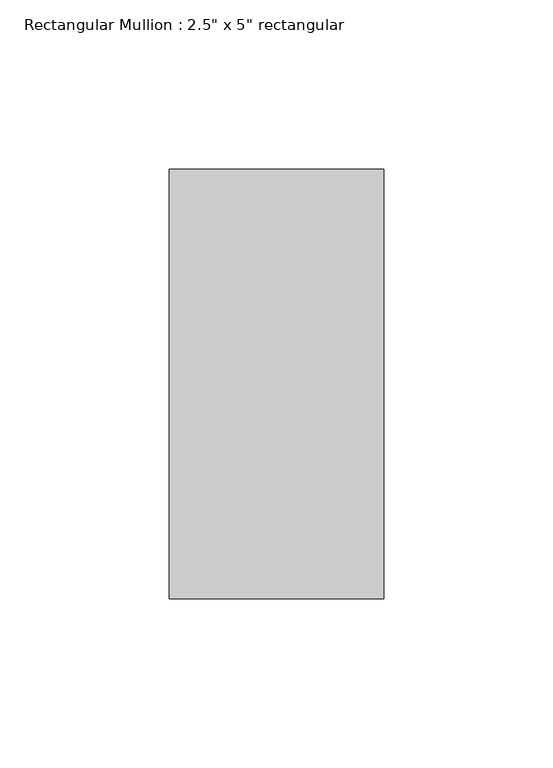
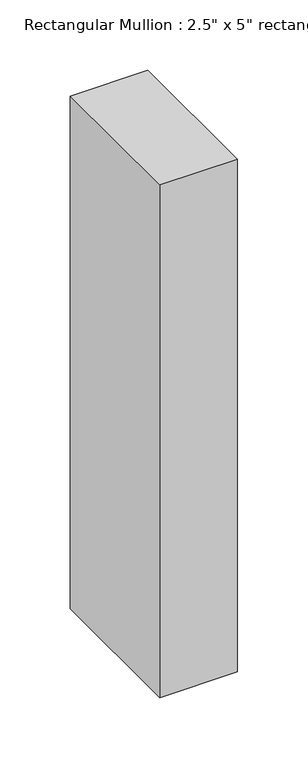
"""IFC4 building model written with IfcOpenShell, lengths in millimetres: member geometry."""

from ifc_helpers import new_model, si_unit, frame, origin, place, context, project, spatial, polyline, outline, extrude, source, transform, mapped, element, save


def member_bc7dbe04(model_context):
    return source(origin(), model_context, "Body", "SweptSolid", [
        extrude(outline(polyline([(0.0, 63.5), (0.0, -63.5), (-63.5, -63.5), (-63.5, 63.5), (0.0, 63.5)])), frame((0.0, 0.0, -444.5), z_axis=(0.0, 0.0, 1.0), x_axis=(1.0, 0.0, 0.0)), (0.0, 0.0, 1.0), 444.5),
    ])


if __name__ == "__main__":
    model = new_model("IFC4")
    model_context = context("Model", 3, world=origin())
    ifc_project = project(units=[si_unit("LENGTHUNIT", "METRE", prefix="MILLI")], contexts=[model_context])
    site = spatial("IfcSite", under=ifc_project)
    building = spatial("IfcBuilding", under=site)
    placement = place(None, origin())
    member_shape = member_bc7dbe04(model_context)
    element("IfcMember", 1, ObjectType="Rectangular Mullion : 2.5\" x 5\" rectangular", at=placement, inside=building, context=model_context, shape_type="MappedRepresentation", body=[
        mapped(member_shape, transform((0.0, 0.0, 0.0), x_axis=(1.0, 0.0, 0.0), y_axis=(0.0, 1.0, 0.0), z_axis=(0.0, 0.0, 1.0))),
    ])
    save(model, "model.ifc")

# Revit data of these elements
# Type "Rectangular Mullion : 2.5\" x 5\" rectangular"
#   built-in parameter 1007304 = 0.416667 (stored number, unit not read)
#   built-in parameter 1007301 = 0.104167 (stored number, unit not read)
#   built-in parameter 1007300 = 0.104167 (stored number, unit not read)
